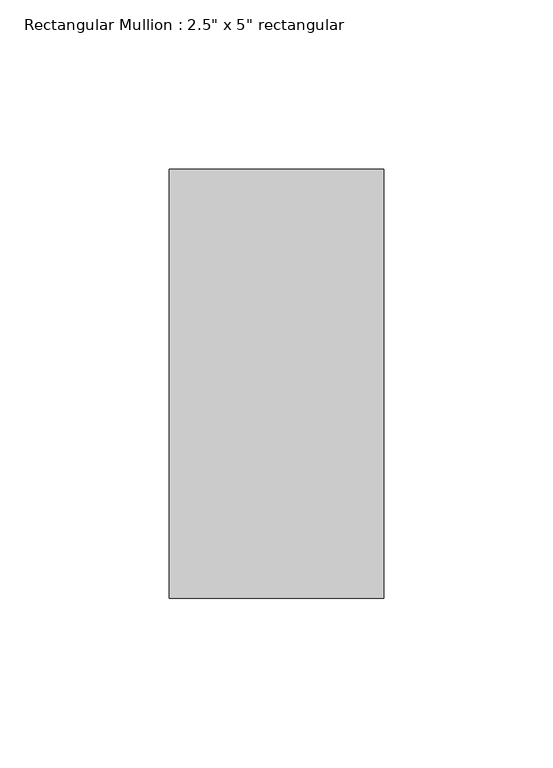
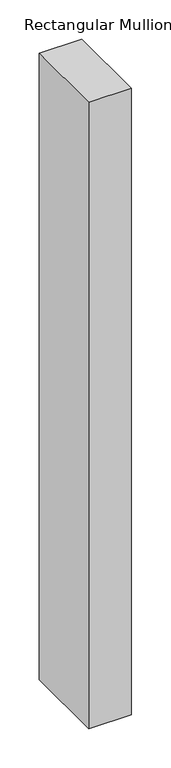
"""IFC4 building model written with IfcOpenShell, lengths in millimetres: member geometry."""

from ifc_helpers import new_model, si_unit, frame, origin, place, context, project, spatial, polyline, outline, extrude, source, transform, mapped, element, save


def member_66f327b8(model_context):
    return source(origin(), model_context, "Body", "SweptSolid", [
        extrude(outline(polyline([(31.75, 63.5), (31.75, -63.5), (-31.75, -63.5), (-31.75, 63.5), (31.75, 63.5)])), frame((0.0, 0.0, -980.0145651), z_axis=(0.0, 0.0, 1.0), x_axis=(1.0, 0.0, 0.0)), (0.0, 0.0, 1.0), 980.0145651),
    ])


if __name__ == "__main__":
    model = new_model("IFC4")
    model_context = context("Model", 3, world=origin())
    ifc_project = project(units=[si_unit("LENGTHUNIT", "METRE", prefix="MILLI")], contexts=[model_context])
    site = spatial("IfcSite", under=ifc_project)
    building = spatial("IfcBuilding", under=site)
    placement = place(None, origin())
    member_shape = member_66f327b8(model_context)
    element("IfcMember", 1, ObjectType="Rectangular Mullion : 2.5\" x 5\" rectangular", at=placement, inside=building, context=model_context, shape_type="MappedRepresentation", body=[
        mapped(member_shape, transform((0.0, 0.0, 0.0), x_axis=(1.0, 0.0, 0.0), y_axis=(0.0, 1.0, 0.0), z_axis=(0.0, 0.0, 1.0))),
    ])
    save(model, "model.ifc")

# Revit data of these elements
# Type "Rectangular Mullion : 2.5\" x 5\" rectangular"
#   built-in parameter 1007304 = 0.416667 (stored number, unit not read)
#   built-in parameter 1007301 = 0.104167 (stored number, unit not read)
#   built-in parameter 1007300 = 0.104167 (stored number, unit not read)
# Element 1 (IfcMember, "Rectangular Mullion : 2.5\" x 5\" rectangular")
#   Materials on its faces: "Aluminum"
# Materials
#   "Aluminum": class "Metal", colour RGB 247 247 247, transparency 0, Description = "Aluminum 6061", Cost = 0
